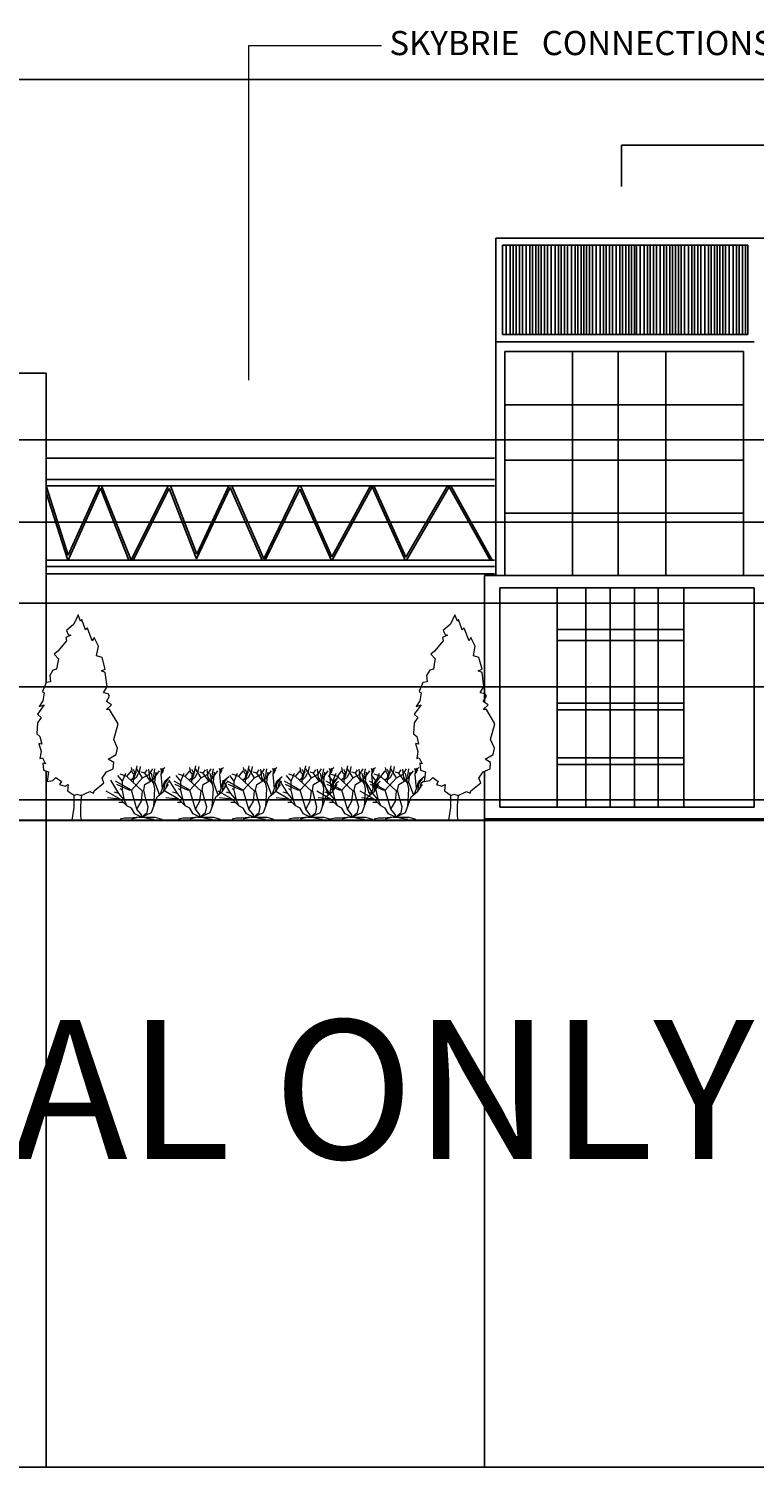
# Model space of a CAD drawing. Units: inches. Extents: x -32109 to 33221, y -19197 to 7608.
# Tile 17 of 25: x -741 to 2967, y -5430 to 1922. Entities that reach past the tile are written whole.
import ezdxf

# ---------------------------------------------------------------- set-up
doc = ezdxf.new("R2010")
doc.units = ezdxf.units.IN
doc.header["$MEASUREMENT"] = 0
for name, color, linetype, lineweight in [('A-ANNO-DIMS', 2, 'Continuous', 18), ('A-ANNO-NOTE', 2, 'Continuous', 18), ('A-ANNO-TEXT', 7, 'Continuous', 25), ('A-ELEV', 7, 'Continuous', 25), ('L-PLNT', 3, 'Continuous', 13)]:
    doc.layers.add(name, color=color, linetype=linetype, lineweight=lineweight)
doc.styles.get("Standard").update_dxf_attribs({"font": 'arial.ttf'})
doc.dimstyles.get("Standard").update_dxf_attribs({"dimtxt": 0.18, "dimasz": 0.18, "dimexe": 0.18, "dimexo": 0.0625, "dimgap": 0.09, "dimtad": 0, "dimtih": 1, "dimtoh": 1, "dimdec": 4, "dimzin": 0, "dimdsep": 46, "dimtxsty": 'Standard', "dimcen": 0.09, "dimadec": 0, "dimazin": 0, "dimtfac": 1, "dimtdec": 4, "dimtofl": 0, "dimtmove": 0, "dimatfit": 3, "dimfxl": 1, "dimtolj": 1, "dimtzin": 0, "dimarcsym": 0})

# ---------------------------------------------------------------- blocks, each defined once
blk = doc.blocks.new('*U2')
blk.add_lwpolyline([(-2.75400000000036, 191.699), (-6.7800000000002, 182.8509999999996), (-13.68200000000024, 176.9529999999995), (-11.95600000000013, 173.2659999999996), (-9.655999999999949, 172.529), (-14.25700000000006, 170.317), (-13.68200000000024, 167.3679999999999), (-21.73300000000017, 157.7829999999999), (-25.1840000000002, 154.8340000000003), (-21.15800000000036, 150.4099999999998), (-21.73300000000017, 147.4609999999998), (-22.88400000000001, 140.8249999999998), (-26.33400000000029, 140.087), (-29.21000000000004, 134.9259999999995), (-28.63499999999977, 129.0279999999998), (-32.66100000000006, 128.2909999999997), (-36.11099999999988, 120.1799999999998), (-34.38599999999997, 118.7059999999997), (-35.53600000000006, 111.3329999999996), (-38.98700000000008, 106.1709999999998), (-34.38599999999997, 107.6459999999997), (-40.71199999999999, 98.79799999999977), (-37.26099999999997, 95.8489999999997), (-40.71199999999999, 90.68799999999965), (-41.28700000000026, 80.36599999999999), (-38.41200000000026, 78.154), (-36.68600000000015, 70.78099999999995), (-39.5619999999999, 71.51799999999957), (-37.26099999999997, 64.14499999999998), (-38.41200000000026, 57.50899999999956), (-36.11099999999988, 58.24699999999984), (-33.23599999999988, 52.3479999999995), (-35.53600000000006, 53.08599999999978), (-34.96100000000024, 46.44999999999981), (-30.36000000000013, 44.9749999999999), (-31.50999999999977, 36.1279999999997), (-26.33400000000029, 36.86499999999978), (-23.45900000000029, 39.81399999999985), (-18.28300000000036, 36.1279999999997), (-20.00800000000027, 33.17799999999988), (-14.83199999999988, 31.70399999999972), (-11.95600000000013, 33.17799999999988), (-12.53099999999995, 27.27999999999975), (-6.204999999999927, 22.85599999999977), (-3.9050000000002, 24.33099999999968), (0.1209999999996398, 22.85599999999977), (8.172999999999774, 26.54299999999967), (11.62399999999979, 25.06799999999976), (12.19900000000007, 27.27999999999975), (21.40000000000009, 34.6529999999998), (19.67500000000018, 39.07699999999977), (23.70099999999957, 44.9749999999999), (30.02700000000004, 47.92399999999997), (30.60199999999986, 53.82299999999986), (25.42599999999993, 56.77199999999993), (32.90299999999979, 61.19599999999991), (34.05299999999988, 67.0939999999996), (30.60199999999986, 75.20499999999993), (34.6279999999997, 89.95100000000002), (26.57599999999957, 103.2219999999997), (23.70099999999957, 103.2219999999997), (28.30199999999968, 107.6459999999997), (23.70099999999957, 110.5949999999998), (26.57599999999957, 115.7559999999994), (25.42599999999993, 117.9679999999998), (20.82499999999982, 118.7059999999997), (24.27599999999984, 124.6040000000002), (22.55099999999993, 137.8759999999997), (19.09999999999991, 139.3499999999999), (22.55099999999993, 140.8249999999998), (19.67500000000018, 151.884), (14.49899999999979, 153.3589999999999), (16.22400000000016, 162.2069999999999), (12.19900000000007, 170.317), (10.47299999999995, 167.3679999999999), (5.871999999999843, 179.1649999999999), (4.146999999999934, 177.69), (0.6959999999999127, 187.2749999999996), (-0.4540000000001783, 185.7999999999997)], close=True)
for points in [[(-6.813000000000101, 23.66899999999987), (-6.813000000000101, 11.66899999999987), (-8.626999999999953, 0)], [(0.3869999999997162, 23.66899999999987), (-0.5760000000000219, 13.27099999999973), (-0.5760000000000219, 3.685999999999694), (0, 0)]]:
    blk.add_lwpolyline(points)
blk = doc.blocks.new('*U3')
for p, q in [((-16.79999999999995, 16.31999999999993), (-18.7199999999998, 18.7199999999998)), ((-14.87999999999988, 18.24000000000001), (-17.75999999999999, 19.19999999999982)), ((-16.79999999999995, 16.31999999999993), (-15.3599999999999, 19.67999999999983)), ((-14.87999999999988, 18.24000000000001), (-12.95999999999981, 20.63999999999987)), ((-12.47099999999977, 19.77499999999986), (-12.89799999999991, 22.04399999999987)), ((-11.67699999999991, 19.07099999999991), (-12.47099999999977, 19.77499999999986)), ((-11.27999999999997, 19.61899999999991), (-12.10400000000004, 21.18399999999974)), ((-12.04299999999989, 15.6279999999997), (-11.92099999999982, 18.83600000000001)), ((-11.92099999999982, 18.83600000000001), (-10.6400000000001, 20.40100000000007)), ((-11.43299999999999, 18.28899999999976), (-10.45699999999988, 22.7489999999998)), ((-10.57899999999995, 18.05399999999986), (-9.845999999999776, 19.69699999999966)), ((-8.160000000000082, 17.75999999999999), (-10.55999999999994, 21.59999999999991)), ((-9.480000000000018, 19.77499999999986), (-8.991999999999962, 22.59199999999964)), ((-7.200000000000045, 19.67999999999983), (-8.6400000000001, 20.15999999999985)), ((-8.160000000000082, 17.75999999999999), (-5.279999999999972, 19.19999999999982)), ((-7.200000000000045, 19.67999999999983), (-6.240000000000009, 21.11999999999989)), ((-4.799999999999954, 16.31999999999993), (-7.200000000000045, 19.67999999999983)), ((-5.085999999999785, 17.74099999999998), (-5.512999999999919, 21.33999999999992)), ((-5.279999999999972, 19.19999999999982), (-3.840000000000145, 21.59999999999991)), ((-2.880000000000109, 12.95999999999981), (-4.319999999999936, 19.67999999999983)), ((-3.840000000000145, 16.79999999999995), (-0.9600000000000363, 20.63999999999987)), ((-3.376999999999952, 18.60199999999963), (-2.887999999999919, 21.57499999999982)), ((-2.765999999999849, 16.80199999999968), (-3.376999999999952, 18.60199999999963)), ((-2.880000000000109, 15.83999999999992), (-2.40000000000009, 20.15999999999985)), ((-0.5079999999998109, 21.88799999999969), (-0.0809999999999036, 20.55799999999976)), ((-0.2029999999999745, 19.14899999999988), (0.1020000000000891, 21.33999999999992)), ((0.3460000000000036, 13.20299999999974), (-0.2029999999999745, 19.14899999999988)), ((-0.1419999999998254, 19.38399999999979), (0.5899999999999181, 20.40100000000007)), ((-0.0199999999999818, 20.00999999999999), (0.895999999999958, 21.10499999999979)), ((0.04099999999994, 20.71399999999994), (1.384000000000241, 22.04399999999987)), ((0.1020000000000891, 21.33999999999992), (0.8350000000000363, 21.88799999999969)), ((-18.23999999999978, 11.03999999999996), (-21.75499999999988, 16.65499999999997)), ((-12.95999999999981, 12.47999999999979), (-19.67999999999983, 16.31999999999993)), ((-13.91999999999984, 12.47999999999979), (-19.19999999999982, 14.87999999999988)), ((-16.79999999999995, 12.47999999999979), (-17.75999999999999, 12.95999999999981)), ((-16.79999999999995, 12.47999999999979), (-16.79999999999995, 16.31999999999993)), ((-15.83999999999992, 8.159999999999854), (-16.79999999999995, 12.47999999999979)), ((-8.160000000000082, 12), (-14.87999999999988, 18.24000000000001)), ((-12.95999999999981, 12.47999999999979), (-13.91999999999984, 12.47999999999979)), ((-13.32499999999982, 16.72399999999993), (-11.43299999999999, 18.28899999999976)), ((-12.95999999999981, 12.47999999999979), (-8.160000000000082, 17.75999999999999)), ((-10.55999999999994, 4.319999999999936), (-12.95999999999981, 12.47999999999979)), ((-11.98199999999997, 16.80199999999968), (-10.57899999999995, 18.05399999999986)), ((-7.680000000000063, 12.47999999999979), (-7.200000000000045, 14.87999999999988)), ((-6.720000000000027, 8.639999999999873), (-7.680000000000063, 12.47999999999979)), ((-7.200000000000045, 14.87999999999988), (-3.840000000000145, 16.79999999999995)), ((-3.376999999999952, 15.31499999999982), (-5.085999999999785, 17.81899999999973)), ((-3.360000000000127, 5.279999999999972), (-2.880000000000109, 12.95999999999981)), ((-0.9600000000000363, 10.55999999999994), (-2.880000000000109, 15.83999999999992)), ((-0.4800000000000182, 10.79999999999995), (0.3460000000000036, 13.20299999999974)), ((0.3460000000000036, 13.20299999999974), (1.323000000000092, 16.2539999999999)), ((0.9600000000000363, 12), (1.440000000000054, 15.3599999999999)), ((0.9600000000000363, 12), (2.879999999999881, 14.87999999999988)), ((1.323000000000092, 16.2539999999999), (3.642000000000052, 18.28899999999976)), ((1.440000000000054, 15.3599999999999), (2.879999999999881, 17.27999999999997)), ((1.920000000000072, 13.43999999999982), (2.399999999999863, 15.3599999999999)), ((2.399999999999863, 15.3599999999999), (3.359999999999899, 16.31999999999993)), ((-17.75999999999999, 8.639999999999873), (-23.66300000000001, 11.96100000000001)), ((-17.75999999999999, 8.639999999999873), (-23.12799999999993, 9.221999999999753)), ((-18.23999999999978, 11.03999999999996), (-20.15999999999985, 11.51999999999998)), ((-15.83999999999992, 8.159999999999854), (-18.23999999999978, 11.03999999999996)), ((-16.31999999999993, 7.199999999999818), (-18.23999999999978, 7.199999999999818)), ((-14.87999999999988, 5.75999999999999), (-17.75999999999999, 8.639999999999873)), ((-14.87999999999988, 5.75999999999999), (-15.83999999999992, 8.159999999999854)), ((-10.55999999999994, 4.319999999999936), (-8.6400000000001, 7.679999999999836)), ((-8.6400000000001, 7.679999999999836), (-8.160000000000082, 12)), ((-5.75999999999999, 5.279999999999972), (-6.720000000000027, 8.639999999999873)), ((-4.319999999999936, 2.879999999999881), (-1.920000000000072, 9.599999999999909)), ((-1.920000000000072, 9.599999999999909), (0.9600000000000363, 12)), ((-15.83999999999992, 0.4799999999997909), (-17.75999999999999, 0)), ((-13.43999999999982, 0.4799999999997909), (-15.83999999999992, 0.4799999999997909)), ((-12.95999999999981, 4.799999999999954), (-14.87999999999988, 5.75999999999999)), ((-9.600000000000136, 0.959999999999809), (-13.43999999999982, 0.4799999999997909)), ((-11.51999999999998, 2.399999999999863), (-12.95999999999981, 4.799999999999954)), ((-9.600000000000136, 0.959999999999809), (-12.95999999999981, 0)), ((-8.6400000000001, 0.959999999999809), (-11.51999999999998, 2.399999999999863)), ((-8.6400000000001, 1.919999999999845), (-10.55999999999994, 4.319999999999936)), ((-9.600000000000136, 0.959999999999809), (-7.680000000000063, 0.959999999999809)), ((-8.6400000000001, 0.959999999999809), (-4.319999999999936, 2.879999999999881)), ((-8.6400000000001, 0.959999999999809), (-6.240000000000009, 2.879999999999881)), ((-8.6400000000001, 0.959999999999809), (-8.6400000000001, 1.919999999999845)), ((-8.6400000000001, 0.959999999999809), (-2.880000000000109, 0.959999999999809)), ((-7.680000000000063, 0.959999999999809), (-6.240000000000009, 0.4799999999997909)), ((-6.240000000000009, 2.879999999999881), (-5.75999999999999, 5.279999999999972)), ((-6.240000000000009, 0.4799999999997909), (-3.360000000000127, 0)), ((-2.880000000000109, 0.959999999999809), (0, 0))]:
    blk.add_line(p, q)
blk = doc.blocks.new('*D10')
at = {"layer": 'A-ANNO-DIMS', "color": 0, "lineweight": -2, "transparency": 16777216}
for p, q in [((-18512.646816, -110.179138), (-18512.646816, 5772.015489000001)), ((-18512.466816, 5771.835489), (-202.0927503703958, 5771.835489)), ((18109.136745, 5771.835489), (-201.2373206296045, 5771.835489)), ((18109.316745, -101.537382), (18109.316745, 5772.015489000001))]:
    blk.add_line(p, q, dxfattribs=at)
at = {"layer": 'A-ANNO-DIMS', "color": 0, "transparency": 16777216}
for points in [[(-18512.466816, 5771.865488999999), (-18512.466816, 5771.805489000001), (-18512.646816, 5771.835489)], [(18109.136745, 5771.865488999999), (18109.136745, 5771.805489000001), (18109.316745, 5771.835489)]]:
    blk.add_solid(points, dxfattribs=at)
at = {"layer": 'Defpoints', "color": 0, "transparency": 16777216}
for p in [(18109.316745, 5771.835489), (-18512.646816, -110.241638), (18109.316745, -101.599882)]:
    blk.add_point(p, dxfattribs=at)
at = {"layer": 'A-ANNO-DIMS', "color": 0, "transparency": 16777216, "insert": (-201.6650355000002, 5771.835489), "char_height": 0.18, "attachment_point": 5}
blk.add_mtext('\\A1;36622', dxfattribs=at)
blk = doc.blocks.new('*D11')
at = {"layer": 'A-ANNO-DIMS', "color": 0, "lineweight": -2, "transparency": 16777216}
for p, q in [((14509.612941, 1705.161904000001), (25710.64858400003, 1705.161904000003)), ((25710.46858400003, 1704.981904000003), (25710.46858400003, -209.6323674706641)), ((25710.46858400003, -2124.610567999994), (25710.46858400003, -209.9962965293272)), ((-18512.58431600001, -2124.790568000001), (25710.64858400003, -2124.790567999994))]:
    blk.add_line(p, q, dxfattribs=at)
at = {"layer": 'A-ANNO-DIMS', "color": 0, "transparency": 16777216}
for points in [[(25710.43858400003, 1704.981904000003), (25710.49858400002, 1704.981904000003), (25710.46858400003, 1705.161904000003)], [(25710.43858400003, -2124.610567999994), (25710.49858400002, -2124.610567999994), (25710.46858400003, -2124.790567999994)]]:
    blk.add_solid(points, dxfattribs=at)
at = {"layer": 'Defpoints', "color": 0, "transparency": 16777216}
for p in [(14509.550441, 1705.161904000001), (-18512.64681600001, -2124.790568000001), (25710.46858400003, -2124.790567999994)]:
    blk.add_point(p, dxfattribs=at)
at = {"layer": 'A-ANNO-DIMS', "color": 0, "transparency": 16777216, "insert": (25710.46858400002, -209.8143320000029), "char_height": 0.18, "attachment_point": 5}
blk.add_mtext('\\A1;3830', dxfattribs=at)
blk = doc.blocks.new('*D12')
at = {"layer": 'A-ANNO-DIMS', "color": 0, "lineweight": -2, "transparency": 16777216}
for p, q in [((-650.959276, -2124.853068), (-650.9592760000002, -5429.734913)), ((1588.180692, -2116.211312), (1588.180692, -5429.734913)), ((-650.7792760000003, -5429.554913), (468.2502168676667, -5429.554913)), ((1588.000691999999, -5429.554913), (468.9711991323325, -5429.554913))]:
    blk.add_line(p, q, dxfattribs=at)
at = {"layer": 'A-ANNO-DIMS', "color": 0, "transparency": 16777216}
for points in [[(-650.7792760000003, -5429.524913), (-650.7792760000003, -5429.584913), (-650.9592760000002, -5429.554913)], [(1588.000691999999, -5429.524913), (1588.000691999999, -5429.584913), (1588.180692, -5429.554913)]]:
    blk.add_solid(points, dxfattribs=at)
at = {"layer": 'Defpoints', "color": 0, "transparency": 16777216}
for p in [(-650.959276, -2124.790568), (1588.180692, -2116.148812), (1588.180692, -5429.554913)]:
    blk.add_point(p, dxfattribs=at)
at = {"layer": 'A-ANNO-DIMS', "color": 0, "transparency": 16777216, "insert": (468.6107079999996, -5429.554913), "char_height": 0.18, "attachment_point": 5}
blk.add_mtext('\\A1;2239', dxfattribs=at)
blk = doc.blocks.new('*D31')
at = {"layer": 'A-ANNO-DIMS', "color": 0, "lineweight": -2, "transparency": 16777216}
for p, q in [((-3370.568291, -2124.853068), (-3370.568291, -5429.734913)), ((-650.959276, -2124.853068), (-650.9592760000002, -5429.734913)), ((-3370.388291000001, -5429.554913), (-2011.228885819236, -5429.554913)), ((-651.1392760000002, -5429.554913), (-2010.298681180764, -5429.554913))]:
    blk.add_line(p, q, dxfattribs=at)
at = {"layer": 'A-ANNO-DIMS', "color": 0, "transparency": 16777216}
for points in [[(-3370.388291000001, -5429.524913), (-3370.388291000001, -5429.584913), (-3370.568291, -5429.554913)], [(-651.1392760000002, -5429.524913), (-651.1392760000002, -5429.584913), (-650.9592760000002, -5429.554913)]]:
    blk.add_solid(points, dxfattribs=at)
at = {"layer": 'Defpoints', "color": 0, "transparency": 16777216}
for p in [(-3370.568291, -2124.790568), (-650.959276, -2124.790568), (-650.9592760000002, -5429.554913)]:
    blk.add_point(p, dxfattribs=at)
at = {"layer": 'A-ANNO-DIMS', "color": 0, "transparency": 16777216, "insert": (-2010.7637835, -5429.554913), "char_height": 0.18, "attachment_point": 5}
blk.add_mtext('\\A1;2719.6', dxfattribs=at)
blk = doc.blocks.new('*D41')
at = {"layer": 'A-ANNO-DIMS', "color": 0, "lineweight": -2, "transparency": 16777216}
for p, q in [((-651.0217760000003, 162.185712), (-24361.99565300002, 162.1857119999962)), ((-24361.81565300002, 162.0057119999962), (-24361.81565300002, -981.1205248622146)), ((-24361.81565300002, -2124.610568000005), (-24361.81565300002, -981.4843311377945)), ((-651.0217760000003, -2124.790568000001), (-24361.99565300002, -2124.790568000005))]:
    blk.add_line(p, q, dxfattribs=at)
at = {"layer": 'A-ANNO-DIMS', "color": 0, "transparency": 16777216}
for points in [[(-24361.84565300001, 162.0057119999962), (-24361.78565300002, 162.0057119999962), (-24361.81565300002, 162.1857119999962)], [(-24361.84565300001, -2124.610568000005), (-24361.78565300002, -2124.610568000005), (-24361.81565300002, -2124.790568000005)]]:
    blk.add_solid(points, dxfattribs=at)
at = {"layer": 'Defpoints', "color": 0, "transparency": 16777216}
for p in [(-650.9592760000002, 162.185712), (-24361.81565300002, -2124.790568000005), (-650.9592760000002, -2124.790568000001)]:
    blk.add_point(p, dxfattribs=at)
at = {"layer": 'A-ANNO-DIMS', "color": 0, "transparency": 16777216, "insert": (-24361.81565300001, -981.3024279999973), "char_height": 0.18, "attachment_point": 5}
blk.add_mtext('\\A1;2287', dxfattribs=at)
blk = doc.blocks.new('*D53')
at = {"layer": 'A-ANNO-DIMS', "color": 0, "lineweight": -2, "transparency": 16777216}
for p, q in [((-9508.270603000004, -179.678781), (25710.64858400002, -179.6787809999944)), ((25710.46858400003, -179.8587809999944), (25710.46858400003, -389.7342653622047)), ((25710.46858400003, -599.9735559999946), (25710.46858400003, -390.0980716377845)), ((-9508.270603000004, -600.1535560000002), (25710.64858400002, -600.1535559999945))]:
    blk.add_line(p, q, dxfattribs=at)
at = {"layer": 'A-ANNO-DIMS', "color": 0, "transparency": 16777216}
for points in [[(25710.43858400003, -179.8587809999944), (25710.49858400002, -179.8587809999944), (25710.46858400003, -179.6787809999944)], [(25710.43858400003, -599.9735559999946), (25710.49858400002, -599.9735559999946), (25710.46858400003, -600.1535559999945)]]:
    blk.add_solid(points, dxfattribs=at)
at = {"layer": 'Defpoints', "color": 0, "transparency": 16777216}
for p in [(-9508.333103000004, -179.678781), (-9508.333103000004, -600.1535560000002), (25710.46858400003, -600.1535559999945)]:
    blk.add_point(p, dxfattribs=at)
at = {"layer": 'A-ANNO-DIMS', "color": 0, "transparency": 16777216, "insert": (25710.46858400002, -389.9161685000017), "char_height": 0.18, "attachment_point": 5}
blk.add_mtext('\\A1;420.5', dxfattribs=at)
blk = doc.blocks.new('*D54')
at = {"layer": 'A-ANNO-DIMS', "color": 0, "lineweight": -2, "transparency": 16777216}
for p, q in [((-9508.270603000004, -600.1535560000002), (25710.64858400002, -600.1535559999945)), ((25710.46858400003, -600.3335559999944), (25710.46858400003, -806.8386914706632)), ((25710.46858400003, -1013.707755999995), (25710.46858400003, -807.2026205293262)), ((-9508.270603000004, -1013.887756), (25710.64858400002, -1013.887755999995))]:
    blk.add_line(p, q, dxfattribs=at)
at = {"layer": 'A-ANNO-DIMS', "color": 0, "transparency": 16777216}
for points in [[(25710.43858400003, -600.3335559999944), (25710.49858400002, -600.3335559999944), (25710.46858400003, -600.1535559999945)], [(25710.43858400003, -1013.707755999995), (25710.49858400002, -1013.707755999995), (25710.46858400003, -1013.887755999995)]]:
    blk.add_solid(points, dxfattribs=at)
at = {"layer": 'Defpoints', "color": 0, "transparency": 16777216}
for p in [(-9508.333103000004, -600.1535560000002), (-9508.333103000004, -1013.887756), (25710.46858400003, -1013.887755999995)]:
    blk.add_point(p, dxfattribs=at)
at = {"layer": 'A-ANNO-DIMS', "color": 0, "transparency": 16777216, "insert": (25710.46858400002, -807.0206560000016), "char_height": 0.18, "attachment_point": 5}
blk.add_mtext('\\A1;413.7', dxfattribs=at)
blk = doc.blocks.new('*D55')
at = {"layer": 'A-ANNO-DIMS', "color": 0, "lineweight": -2, "transparency": 16777216}
for p, q in [((-9508.270603000004, -1013.887756), (25710.64858400002, -1013.887755999995)), ((25710.46858400003, -1014.067755999994), (25710.46858400003, -1227.669337362204)), ((25710.46858400003, -1441.634724999994), (25710.46858400003, -1228.033143637784)), ((-9508.270603000004, -1441.814725), (25710.64858400002, -1441.814724999995))]:
    blk.add_line(p, q, dxfattribs=at)
at = {"layer": 'A-ANNO-DIMS', "color": 0, "transparency": 16777216}
for points in [[(25710.43858400003, -1014.067755999994), (25710.49858400002, -1014.067755999994), (25710.46858400003, -1013.887755999995)], [(25710.43858400003, -1441.634724999994), (25710.49858400002, -1441.634724999994), (25710.46858400003, -1441.814724999995)]]:
    blk.add_solid(points, dxfattribs=at)
at = {"layer": 'Defpoints', "color": 0, "transparency": 16777216}
for p in [(-9508.333103000004, -1013.887756), (-9508.333103000004, -1441.814725), (25710.46858400003, -1441.814724999995)]:
    blk.add_point(p, dxfattribs=at)
at = {"layer": 'A-ANNO-DIMS', "color": 0, "transparency": 16777216, "insert": (25710.46858400002, -1227.851240500001), "char_height": 0.18, "attachment_point": 5}
blk.add_mtext('\\A1;427.9', dxfattribs=at)
blk = doc.blocks.new('*D56')
at = {"layer": 'A-ANNO-DIMS', "color": 0, "lineweight": -2, "transparency": 16777216}
for p, q in [((-9508.270603000004, -1441.814725), (25710.64858400002, -1441.814724999995)), ((25710.46858400003, -1441.994724999995), (25710.46858400003, -1730.102620862205)), ((25710.46858400003, -2018.574322999995), (25710.46858400003, -1730.466427137785)), ((-9508.270603000004, -2018.754323000001), (25710.64858400002, -2018.754322999996))]:
    blk.add_line(p, q, dxfattribs=at)
at = {"layer": 'A-ANNO-DIMS', "color": 0, "transparency": 16777216}
for points in [[(25710.43858400003, -1441.994724999995), (25710.49858400002, -1441.994724999995), (25710.46858400003, -1441.814724999995)], [(25710.43858400003, -2018.574322999995), (25710.49858400002, -2018.574322999995), (25710.46858400003, -2018.754322999996)]]:
    blk.add_solid(points, dxfattribs=at)
at = {"layer": 'Defpoints', "color": 0, "transparency": 16777216}
for p in [(-9508.333103000004, -1441.814725), (-9508.333103000004, -2018.754323000001), (25710.46858400003, -2018.754322999996)]:
    blk.add_point(p, dxfattribs=at)
at = {"layer": 'A-ANNO-DIMS', "color": 0, "transparency": 16777216, "insert": (25710.46858400002, -1730.284524000002), "char_height": 0.18, "attachment_point": 5}
blk.add_mtext('\\A1;576.9', dxfattribs=at)
blk = doc.blocks.new('*D57')
at = {"layer": 'A-ANNO-DIMS', "color": 0, "lineweight": -2, "transparency": 16777216}
for p, q in [((1588.180692, -2116.211312), (1588.180692, -5429.734913)), ((3022.7376, -2131.466103000001), (3022.7376, -5429.734913)), ((1588.360692, -5429.554913), (2305.004050502047, -5429.554913)), ((3022.5576, -5429.554913), (2305.914241497954, -5429.554913))]:
    blk.add_line(p, q, dxfattribs=at)
at = {"layer": 'A-ANNO-DIMS', "color": 0, "transparency": 16777216}
for points in [[(1588.360692, -5429.524913), (1588.360692, -5429.584913), (1588.180692, -5429.554913)], [(3022.5576, -5429.524913), (3022.5576, -5429.584913), (3022.7376, -5429.554913)]]:
    blk.add_solid(points, dxfattribs=at)
at = {"layer": 'Defpoints', "color": 0, "transparency": 16777216}
for p in [(1588.180692, -2116.148812), (3022.7376, -2131.403603), (3022.7376, -5429.554913)]:
    blk.add_point(p, dxfattribs=at)
at = {"layer": 'A-ANNO-DIMS', "color": 0, "transparency": 16777216, "insert": (2305.459146, -5429.554913), "char_height": 0.18, "attachment_point": 5}
blk.add_mtext('\\A1;1434.6', dxfattribs=at)
blk = doc.blocks.new('*D67')
at = {"layer": 'A-ANNO-DIMS', "color": 0, "lineweight": -2, "transparency": 16777216}
for p, q in [((1645.907271000001, 851.2050040000005), (25710.64858400003, 851.2050040000044)), ((25710.46858400003, 851.0250040000043), (25710.46858400003, -632.2900008622063)), ((25710.46858400003, -2115.968811999997), (25710.46858400003, -632.6538071377862)), ((1588.243192000001, -2116.148812000001), (25710.64858400003, -2116.148811999997))]:
    blk.add_line(p, q, dxfattribs=at)
at = {"layer": 'A-ANNO-DIMS', "color": 0, "transparency": 16777216}
for points in [[(25710.43858400003, 851.0250040000043), (25710.49858400002, 851.0250040000043), (25710.46858400003, 851.2050040000044)], [(25710.43858400003, -2115.968811999997), (25710.49858400002, -2115.968811999997), (25710.46858400003, -2116.148811999997)]]:
    blk.add_solid(points, dxfattribs=at)
at = {"layer": 'Defpoints', "color": 0, "transparency": 16777216}
for p in [(1645.844771000001, 851.2050040000005), (1588.180692, -2116.148812000001), (25710.46858400003, -2116.148811999997)]:
    blk.add_point(p, dxfattribs=at)
at = {"layer": 'A-ANNO-DIMS', "color": 0, "transparency": 16777216, "insert": (25710.46858400002, -632.4719040000035), "char_height": 0.18, "attachment_point": 5}
blk.add_mtext('\\A1;2967.4', dxfattribs=at)
blk = doc.blocks.new('*D158')
at = {"layer": 'A-ANNO-DIMS', "color": 0, "lineweight": -2, "transparency": 16777216}
for p, q in [((5447.266114000002, 1662.169531000001), (-24361.99565300002, 1662.169530999996)), ((-24361.81565300002, 1661.989530999996), (-24361.81565300002, -230.1077594706735)), ((-24361.81565300002, -2122.568979000006), (-24361.81565300002, -230.4716885293365)), ((5279.201554000002, -2122.748979000001), (-24361.99565300002, -2122.748979000006))]:
    blk.add_line(p, q, dxfattribs=at)
at = {"layer": 'A-ANNO-DIMS', "color": 0, "transparency": 16777216}
for points in [[(-24361.84565300001, 1661.989530999996), (-24361.78565300002, 1661.989530999996), (-24361.81565300002, 1662.169530999996)], [(-24361.84565300001, -2122.568979000006), (-24361.78565300002, -2122.568979000006), (-24361.81565300002, -2122.748979000006)]]:
    blk.add_solid(points, dxfattribs=at)
at = {"layer": 'Defpoints', "color": 0, "transparency": 16777216}
for p in [(5447.328614000002, 1662.169531000001), (-24361.81565300002, -2122.748979000006), (5279.264054000002, -2122.748979000001)]:
    blk.add_point(p, dxfattribs=at)
at = {"layer": 'A-ANNO-DIMS', "color": 0, "transparency": 16777216, "insert": (-24361.81565300001, -230.289723999998), "char_height": 0.18, "attachment_point": 5}
blk.add_mtext('\\A1;3784.9', dxfattribs=at)

msp = doc.modelspace()

# ---------------------------------------------------------------- linework, layer by layer
at = {"layer": 'A-ANNO-NOTE'}
for p, q in [((384.7068857151317, 126.0443412497407), (384.7068857151317, 1836.671844469616)), ((384.7068857151317, 1836.671844469616), (1061.319766350323, 1836.671844469616))]:
    msp.add_line(p, q, dxfattribs=at)
at = {"layer": 'A-ELEV'}
for p, q in [((3709.007830620743, 1327.301250283199), (2289.325426198426, 1327.301250283199)), ((2289.325426198426, 1327.301250283199), (2289.325426198426, 1116.520092682098)), ((1645.844771085678, 851.2050040502659), (1645.844771085678, 322.0173392160969)), ((2967.282875926691, 851.2050040502659), (1645.844771085678, 851.2050040502659)), ((1680.402772156563, 816.6042807491536), (1680.402772156563, 359.756051500956)), ((1680.402772156563, 816.6042807491536), (2933.869510806688, 816.6042807491535)), ((1698.536664539008, 359.756051500956), (1698.536664539008, 816.6042807491535)), ((1718.967707319338, 359.756051500956), (1718.967707319338, 816.6042807491535)), ((1735.898866136185, 359.756051500956), (1735.898866136185, 816.6042807491535)), ((1749.75165280856, 359.756051500956), (1749.75165280856, 816.6042807491535)), ((1766.682839630973, 359.756051500956), (1766.682839630973, 816.6042807491535)), ((1782.074840381156, 359.756051500956), (1782.074840381156, 816.6042807491535)), ((1802.084399348036, 359.756051500956), (1802.084399348036, 816.6042807491535)), ((1820.554800248247, 359.756051500956), (1820.554800248247, 816.6042807491535)), ((1834.407586920627, 359.756051500956), (1834.407586920627, 816.6042807491535)), ((1851.33874573747, 359.756051500956), (1851.33874573747, 816.6042807491535)), ((1865.191532409849, 359.756051500956), (1865.191532409849, 816.6042807491535)), ((1879.044319082224, 359.756051500956), (1879.044319082224, 816.6042807491535)), ((1894.436319832403, 359.756051500956), (1894.436319832403, 816.6042807491535)), ((1911.282531359138, 816.6042807491536), (1911.282531359138, 359.756051500956)), ((1929.416423741583, 359.756051500956), (1929.416423741583, 816.6042807491535)), ((1949.847466521912, 359.756051500956), (1949.847466521912, 816.6042807491535)), ((1966.77862533876, 359.756051500956), (1966.77862533876, 816.6042807491535)), ((1980.631412011135, 359.756051500956), (1980.631412011135, 816.6042807491535)), ((1997.562598833547, 359.756051500956), (1997.562598833547, 816.6042807491535)), ((2012.954599583731, 359.756051500956), (2012.954599583731, 816.6042807491535)), ((2032.964158550611, 359.756051500956), (2032.964158550611, 816.6042807491535)), ((2051.434559450823, 359.756051500956), (2051.434559450823, 816.6042807491535)), ((2065.287346123202, 359.756051500956), (2065.287346123202, 816.6042807491535)), ((2082.218504940045, 359.756051500956), (2082.218504940045, 816.6042807491535)), ((2096.071291612425, 359.756051500956), (2096.071291612425, 816.6042807491535)), ((2109.924078284799, 359.756051500956), (2109.924078284799, 816.6042807491535)), ((2125.316079034979, 359.756051500956), (2125.316079034979, 816.6042807491535)), ((2140.623104489479, 816.6042807491536), (2140.623104489479, 359.756051500956)), ((2158.756996871924, 359.756051500956), (2158.756996871924, 816.6042807491535)), ((2179.188039652254, 359.756051500956), (2179.188039652254, 816.6042807491535)), ((2196.119198469101, 359.756051500956), (2196.119198469101, 816.6042807491535)), ((2209.971985141476, 359.756051500956), (2209.971985141476, 816.6042807491535)), ((2226.903171963889, 359.756051500956), (2226.903171963889, 816.6042807491535)), ((2242.295172714072, 359.756051500956), (2242.295172714072, 816.6042807491535)), ((2262.304731680952, 359.756051500956), (2262.304731680952, 816.6042807491535)), ((2280.775132581164, 359.756051500956), (2280.775132581164, 816.6042807491535)), ((2294.627919253543, 359.756051500956), (2294.627919253543, 816.6042807491535)), ((2311.559078070386, 359.756051500956), (2311.559078070386, 816.6042807491535)), ((2325.411864742766, 359.756051500956), (2325.411864742766, 816.6042807491535)), ((2339.26465141514, 359.756051500956), (2339.26465141514, 816.6042807491535)), ((2354.656652165319, 359.756051500956), (2354.656652165319, 816.6042807491535)), ((2365.346063391983, 816.6042807491536), (2365.346063391983, 359.756051500956)), ((2383.479955774429, 359.756051500956), (2383.479955774429, 816.6042807491535)), ((2403.910998554759, 359.756051500956), (2403.910998554759, 816.6042807491535)), ((2420.842157371605, 359.756051500956), (2420.842157371605, 816.6042807491535)), ((2434.694944043981, 359.756051500956), (2434.694944043981, 816.6042807491535)), ((2451.626130866392, 359.756051500956), (2451.626130866392, 816.6042807491535)), ((2467.018131616577, 359.756051500956), (2467.018131616577, 816.6042807491535)), ((2487.027690583456, 359.756051500956), (2487.027690583456, 816.6042807491535)), ((2505.498091483668, 359.756051500956), (2505.498091483668, 816.6042807491535)), ((2519.350878156048, 359.756051500956), (2519.350878156048, 816.6042807491535)), ((2536.282036972891, 359.756051500956), (2536.282036972891, 816.6042807491535)), ((2550.13482364527, 359.756051500956), (2550.13482364527, 816.6042807491535)), ((2563.987610317645, 359.756051500956), (2563.987610317645, 816.6042807491535)), ((2579.379611067824, 359.756051500956), (2579.379611067824, 816.6042807491535)), ((2593.147422444521, 816.6042807491536), (2593.147422444521, 359.756051500956)), ((2611.281314826966, 359.756051500956), (2611.281314826966, 816.6042807491535)), ((2631.712357607296, 359.756051500956), (2631.712357607296, 816.6042807491535)), ((2648.643516424142, 359.756051500956), (2648.643516424142, 816.6042807491535)), ((2662.496303096518, 359.756051500956), (2662.496303096518, 816.6042807491535)), ((2679.427489918931, 359.756051500956), (2679.427489918931, 816.6042807491535)), ((2694.819490669113, 359.756051500956), (2694.819490669113, 816.6042807491535)), ((2714.829049635993, 359.756051500956), (2714.829049635993, 816.6042807491535)), ((2733.299450536206, 359.756051500956), (2733.299450536206, 816.6042807491535)), ((2747.152237208585, 359.756051500956), (2747.152237208585, 816.6042807491535)), ((2764.083396025428, 359.756051500956), (2764.083396025428, 816.6042807491535)), ((2777.936182697807, 359.756051500956), (2777.936182697807, 816.6042807491535)), ((2791.788969370182, 359.756051500956), (2791.788969370182, 816.6042807491535)), ((2807.180970120361, 359.756051500956), (2807.180970120361, 816.6042807491535)), ((2820.948809502633, 816.6042807491536), (2820.948809502633, 359.756051500956)), ((2839.082701885078, 359.756051500956), (2839.082701885078, 816.6042807491535)), ((2859.513744665407, 359.756051500956), (2859.513744665407, 816.6042807491535)), ((2876.444903482255, 359.756051500956), (2876.444903482255, 816.6042807491535)), ((2890.297690154629, 359.756051500956), (2890.297690154629, 816.6042807491535)), ((2907.228876977042, 359.756051500956), (2907.228876977042, 816.6042807491535)), ((2922.620877727225, 359.756051500956), (2922.620877727225, 816.6042807491535)), ((2933.869510806688, 359.756051500956), (2933.869510806688, 816.6042807491535)), ((1645.844771085678, 322.0173392160969), (2967.282875926691, 322.0173392160969)), ((1645.844771085678, 322.0173392160969), (1645.844771085678, -871.5754161552333)), ((1680.402772156563, 359.756051500956), (2933.869510806688, 359.756051500956)), ((1692.327012944353, 272.4501353241304), (2911.516649442584, 272.4501353241304)), ((1692.327012944353, -871.5754161552333), (1692.327012944353, 272.4501353241304)), ((2038.860866345503, -871.5754161552333), (2038.860866345503, 272.4501353241304)), ((2271.152778359327, -871.5754161552333), (2271.152778359327, 272.4501353241304)), ((2514.868862107431, -871.5754161552333), (2514.868862107431, 272.4501353241304)), ((2911.516649442584, 272.4501353241304), (2911.516649442584, -871.5754161552333)), ((-3370.568291181102, 162.1857121999783), (-650.9592756182683, 162.1857121999419)), ((-650.9592756182683, 162.1857121999419), (-650.9592756182683, -1419.76050077207)), ((1692.327012944353, 0.5673298303902073), (2911.516649442584, 0.5673298303902073)), ((1639.527927248928, -272.2120093144895), (-650.9592756182682, -272.2120093144895)), ((1692.327012944353, -282.5306023220849), (2911.516649442584, -282.5306023220849)), ((1639.527927248928, -381.6804259145265), (-650.9592756182682, -381.6804259145265)), ((1639.527927248928, -414.4039019166048), (-650.9592756182828, -414.4039019166048)), ((-538.7758485153026, -767.8922555231657), (-650.9592756182828, -414.4039019166048)), ((-374.5527636016486, -426.8467777747628), (-539.5391310848208, -793.987203587556)), ((-379.9244790970842, -414.4039019166048), (-538.7758485153026, -767.8922555231657)), ((-228.6987924132845, -793.987203587556), (-374.5527636016486, -426.8467777747628)), ((-217.9385709619674, -793.987203587556), (-368.8415040586988, -414.1376413017897)), ((-27.7498320316663, -414.4039019166048), (-217.9385709619674, -793.987203587556)), ((-22.87022483158216, -426.9884021735642), (-206.7535487886634, -793.987203587556)), ((117.0589369067893, -787.8655178195913), (-22.87022483158216, -426.9884021735625)), ((117.9552200489415, -762.5161669319386), (-17.02440410161216, -414.4039019166048)), ((289.4410667391785, -422.2577052681026), (117.0589369067893, -787.8655178195913)), ((282.0882927131606, -414.4039019166048), (117.9552200489415, -762.5161669319396)), ((451.7266751647403, -793.987203587556), (289.4410667391785, -422.2577052681035)), ((459.9655642002471, -787.8655178195913), (296.9237667792476, -414.4039019166048)), ((641.5168562749459, -414.4039019166048), (459.9655642002471, -787.8655178195913)), ((644.2134070125176, -431.729388824131), (468.1086306878133, -793.987203587556)), ((804.7286565089889, -791.9358678456574), (644.2134070125176, -431.729388824131)), ((808.736682087896, -776.3622217201728), (647.4407771157857, -414.4039019166048)), ((1005.643373747109, -414.4039019166048), (808.736682087896, -776.3622217201718)), ((1014.486278847616, -419.0748831438805), (810.5325619641371, -793.987203587556)), ((1183.139599608825, -793.4790363899846), (1014.486278847616, -419.0748831438805)), ((1187.207467876404, -778.1615842519677), (1023.349934389247, -414.4039019166048)), ((1398.686517411886, -414.4039019166048), (1187.207467876404, -778.1615842519677)), ((1407.586035900531, -418.9924417993761), (1189.574047000103, -793.987203587556)), ((1616.747521967452, -793.987203587556), (1407.586035900531, -418.9924417993761)), ((1628.197890213458, -793.987203587556), (1416.477046207292, -414.4039019166048)), ((-540.9858399432851, -793.987203587556), (-650.9592756182683, -447.4625009545853)), ((1692.327012944353, -553.5818205641297), (2911.516649442584, -553.5818205641297)), ((-634.4066790939686, -793.987203587556), (-650.9592756182683, -793.9872035875561)), ((1639.527927248928, -793.987203587556), (-634.4066790939686, -793.987203587556)), ((-634.4066790939686, -826.2291201674687), (-650.9592756182683, -826.229120167469)), ((1639.527927248928, -863.0597253706509), (-650.9592756182682, -863.0597253706509)), ((-634.4066790939686, -826.2291201674687), (1639.527927248928, -826.2291201674687)), ((1588.180691889405, -871.5754161552333), (3034.293504197781, -871.5754161552333)), ((1588.180691889405, -1520.673659219526), (1588.180691889405, -871.5754161552333)), ((1667.479524724192, -2056.233701899126), (1667.479524724192, -934.761095456008)), ((1667.479524724192, -934.761095456008), (1692.327012944353, -934.761095456008)), ((1692.327012944353, -934.761095456008), (1692.327012944353, -934.761095456008)), ((1692.327012944353, -934.761095456008), (2967.067564097586, -934.761095456008)), ((1959.749311536489, -934.761095456008), (1959.749311536489, -2056.233701899126)), ((2105.956165252186, -934.761095456008), (2105.956165252186, -2056.233701899126)), ((2230.620883243052, -934.761095456008), (2230.620883243052, -2056.233701899126)), ((2355.285629239483, -934.761095456008), (2355.285629239483, -2056.233701899126)), ((2475.333153086046, -934.761095456008), (2475.333153086046, -2056.233701899126)), ((2606.923704301721, -934.761095456008), (2606.923704301721, -2056.233701899126)), ((2967.067564097586, -934.761095456008), (2967.067564097586, -2056.233701899126)), ((1959.749311536489, -1148.597883789544), (2606.923704301719, -1148.597883789544)), ((1959.749311536489, -1204.499646112347), (2606.923704301719, -1204.499646112347)), ((1959.749311536489, -1525.003088426533), (2606.923704301719, -1525.003088426533)), ((1588.180691889405, -1557.22667194655), (1588.180691889405, -1551.512497277733)), ((1959.749311536489, -1558.544147961695), (2606.923704301719, -1558.544147961695)), ((1959.749311536489, -1804.511910747946), (2606.923704301719, -1804.511910747946)), ((-650.9592756182683, -1872.454523225513), (-650.9592756182683, -2124.790568085177)), ((1588.180691889405, -2116.148811955302), (1588.180691889405, -1873.318006719478)), ((1959.749311536489, -1838.052959575707), (2606.923704301719, -1838.052959575707)), ((2967.067564097586, -2056.233701899126), (1667.479524724192, -2056.233701899126)), ((-18512.64681618521, -2124.790568085177), (1683.58803657419, -2124.790568085177)), ((3034.293504197781, -2116.148811955302), (1588.180691889405, -2116.148811955302))]:
    msp.add_line(p, q, dxfattribs=at)

# ---------------------------------------------------------------- block references
at = {"layer": 'L-PLNT'}
for name, p, xscale, yscale, zscale in [('*U2', (-473.4243250922772, -2122.295119423421), 5.474302449835042, 5.474302449835042, 5.474302449835042), ('*U2', (1452.491456205065, -2122.295119423421), 5.474302449835042, 5.474302449835042, 5.474302449835042), ('*U3', (-61.09829606859239, -2118.430999141933), 11.97885450539613, 11.97885450539613, 11.97885450539613), ('*U3', (237.7508184315102, -2118.430999141933), 11.97885450539613, 11.97885450539613, 11.97885450539613), ('*U3', (510.9841896358866, -2118.430999141933), 11.97885450539613, 11.97885450539613, 11.97885450539613), ('*U3', (801.294600642419, -2118.430999141933), 11.97885450539613, 11.97885450539613, 11.97885450539613), ('*U3', (1014.758332539279, -2118.430999141933), 11.97885450539613, 11.97885450539613, 11.97885450539613), ('*U3', (1236.760400744724, -2118.430999141933), 11.97885450539613, 11.97885450539613, 11.97885450539613)]:
    msp.add_blockref(name, p, dxfattribs=dict(at, xscale=xscale, yscale=yscale, zscale=zscale))

# ---------------------------------------------------------------- texts
at = {"layer": 'A-ANNO-TEXT'}
for s, height, p in [('SKYBRIE   CONNECTIONS', 123.5547426012344, (1102.672851028386, 1787.079753092934)), ('MONUMENTAL    FRONT   FACADE    ( CONCEPTUAL ONLY   NO DIMENSIONS )', 709.7949465747753, (-22238.10681632875, -3853.851877923695))]:
    msp.add_text(s, height=height, dxfattribs=at).set_placement(p)

# ---------------------------------------------------------------- dimensions: what is measured, and where the dimension line sits
at = {"layer": 'A-ANNO-DIMS'}
for base, p1, p2, override, picture, middle in [((18109.316745, 5771.835489), (-18512.646816, -110.241638), (18109.316745, -101.599882), {"dimdec": 0, "dimlfac": 1, "dimrnd": 0, "dimzin": 0, "dimdsep": 46, "dimlunit": 2}, '*D10', (-201.6650355000002, 5771.835489)), ((-650.9592760000002, -5429.554913), (-3370.568291, -2124.790568), (-650.959276, -2124.790568), {"dimdec": 1, "dimlfac": 1, "dimrnd": 0, "dimzin": 0, "dimdsep": 46, "dimlunit": 2}, '*D31', (-2010.7637835, -5429.554913)), ((1588.180692, -5429.554913), (-650.959276, -2124.790568), (1588.180692, -2116.148812), {"dimdec": 0, "dimlfac": 1, "dimrnd": 0, "dimzin": 0, "dimdsep": 46, "dimlunit": 2}, '*D12', (468.6107079999996, -5429.554913)), ((3022.7376, -5429.554913), (1588.180692, -2116.148812), (3022.7376, -2131.403603), {"dimdec": 1, "dimlfac": 1, "dimrnd": 0, "dimzin": 0, "dimdsep": 46, "dimlunit": 2}, '*D57', (2305.459146, -5429.554913))]:
    dim = msp.add_linear_dim(base=base, p1=p1, p2=p2, dimstyle='Standard', override=override, dxfattribs=at)
    dim.commit()
    dim.dimension.update_dxf_attribs({"geometry": picture, "text_midpoint": middle})
for base, p1, p2, override, picture, middle in [((25710.46858400003, -2124.790567999994), (14509.550441, 1705.161904), (-18512.646816, -2124.790568), {"dimdec": 0, "dimlfac": 1, "dimrnd": 0, "dimzin": 0, "dimdsep": 46, "dimlunit": 2}, '*D11', (25710.46858400002, -209.8143320000029)), ((-24361.81565300002, -2122.748979000006), (5447.328613999999, 1662.169531), (5279.264054, -2122.748979), {"dimdec": 1, "dimlfac": 1, "dimrnd": 0, "dimzin": 0, "dimdsep": 46, "dimlunit": 2}, '*D158', (-24361.81565300001, -230.289723999998)), ((25710.46858400003, -2116.148811999997), (1645.844771, 851.205004), (1588.180692, -2116.148812), {"dimdec": 1, "dimlfac": 1, "dimrnd": 0, "dimzin": 0, "dimdsep": 46, "dimlunit": 2}, '*D67', (25710.46858400002, -632.4719040000035)), ((-24361.81565300002, -2124.790568000005), (-650.959276, 162.185712), (-650.959276, -2124.790568), {"dimdec": 0, "dimlfac": 1, "dimrnd": 0, "dimzin": 0, "dimdsep": 46, "dimlunit": 2}, '*D41', (-24361.81565300001, -981.3024279999973)), ((25710.46858400003, -600.1535559999945), (-9508.333103, -179.678781), (-9508.333103, -600.1535559999999), {"dimdec": 1, "dimlfac": 1, "dimrnd": 0, "dimzin": 0, "dimdsep": 46, "dimlunit": 2}, '*D53', (25710.46858400002, -389.9161685000017)), ((25710.46858400003, -1013.887755999995), (-9508.333103, -600.1535559999999), (-9508.333103, -1013.887756), {"dimdec": 1, "dimlfac": 1, "dimrnd": 0, "dimzin": 0, "dimdsep": 46, "dimlunit": 2}, '*D54', (25710.46858400002, -807.0206560000016)), ((25710.46858400003, -1441.814724999995), (-9508.333103, -1013.887756), (-9508.333103, -1441.814725), {"dimdec": 1, "dimlfac": 1, "dimrnd": 0, "dimzin": 0, "dimdsep": 46, "dimlunit": 2}, '*D55', (25710.46858400002, -1227.851240500001)), ((25710.46858400003, -2018.754322999996), (-9508.333103, -1441.814725), (-9508.333103, -2018.754323), {"dimdec": 1, "dimlfac": 1, "dimrnd": 0, "dimzin": 0, "dimdsep": 46, "dimlunit": 2}, '*D56', (25710.46858400002, -1730.284524000002))]:
    dim = msp.add_linear_dim(base=base, p1=p1, p2=p2, angle=90, dimstyle='Standard', override=override, dxfattribs=at)
    dim.commit()
    dim.dimension.update_dxf_attribs({"geometry": picture, "text_midpoint": middle})

doc.saveas('drawing.dxf')
